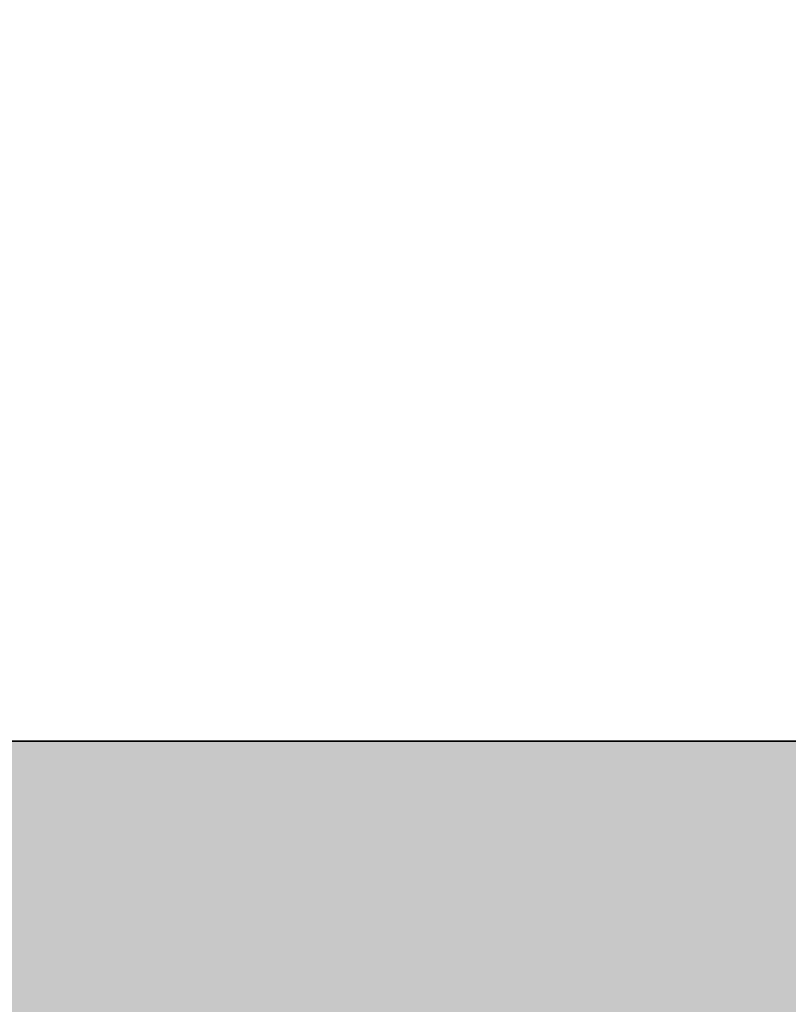
# Model space of a CAD drawing. Units: inches. Extents: x 2696 to 3240, y 1564 to 2310.
# Tile 72 of 76: x 3156.71 to 3168.22, y 2070.76 to 2085.5. Entities that reach past the tile are written whole.
import ezdxf

# ---------------------------------------------------------------- set-up
doc = ezdxf.new("R2010")
doc.units = ezdxf.units.IN
doc.layers.add('A-WALL', color=7, linetype='Continuous', lineweight=35)
doc.layers.add('A-WALL-PATT', color=9, linetype='Continuous', lineweight=13)

msp = doc.modelspace()

# ---------------------------------------------------------------- hatches: boundary and pattern name
at = {"layer": 'A-WALL-PATT', "transparency": 33554556}
h = msp.add_hatch(color=256, dxfattribs=at)
h.dxf.hatch_style = 1
h.paths.add_polyline_path([(2879.111, 2253.201), (2905.91, 2253.201), (2905.91, 2262.201), (2841.889, 2262.201), (2841.889, 2253.201), (2870.111, 2253.201), (2870.111, 2176.601), (2965.709, 2176.601), (2965.709, 2206.701), (2973.583, 2206.701), (2973.583, 2215.701), (2965.709, 2215.701), (2965.709, 2262.201), (2929.91, 2262.201), (2929.91, 2253.201), (2956.709, 2253.201), (2956.709, 2185.601), (2879.111, 2185.601)])
h.paths.add_polyline_path([(2782.834, 2262.201), (2745.611, 2262.201), (2745.611, 2228.729), (2754.611, 2228.729), (2754.611, 2253.201), (2782.834, 2253.201)])
h.paths.add_polyline_path([(2754.611, 2136.201), (2965.709, 2136.201), (2965.709, 2145.201), (2879.111, 2145.201), (2879.111, 2147.074), (2877.34, 2147.074), (2870.111, 2147.074), (2870.111, 2145.201), (2754.611, 2145.201), (2754.611, 2169.674), (2745.611, 2169.674), (2745.611, 2000.201), (2754.611, 2000.201), (2754.611, 2019.201), (2849.083, 2019.201), (2849.083, 2023.701), (2841.209, 2023.701), (2841.209, 2051.827), (2836.709, 2051.827), (2836.709, 2023.701), (2754.611, 2023.701), (2754.611, 2091.201), (2836.709, 2091.201), (2836.709, 2087.827), (2841.209, 2087.827), (2841.209, 2095.701), (2754.611, 2095.701)])
h.paths.add_polyline_path([(2965.709, 2136.201), (2956.709, 2136.201), (2956.709, 2023.701), (2885.083, 2023.701), (2885.083, 2019.201), (2956.709, 2019.201), (2956.709, 1950.575), (2965.709, 1950.575), (2965.709, 1980.201), (2973.583, 1980.201), (2973.583, 1989.201), (2965.709, 1989.201)])
h.paths.add_polyline_path([(2754.611, 1906.701), (2880.209, 1906.701), (2884.709, 1906.701), (2956.709, 1906.701), (2956.709, 1792.701), (2944.709, 1792.701), (2944.709, 1783.701), (2956.709, 1783.701), (2956.709, 1740.201), (2884.709, 1740.201), (2884.709, 1783.701), (2896.709, 1783.701), (2896.709, 1792.701), (2884.709, 1792.701), (2884.709, 1846.701), (2880.209, 1846.701), (2880.209, 1740.201), (2754.611, 1740.201), (2754.611, 1777.201), (2745.611, 1777.201), (2745.611, 1692.701), (2754.611, 1692.701), (2754.611, 1731.201), (2956.709, 1731.201), (2956.709, 1723.327), (2965.709, 1723.327), (2965.709, 1884.201), (2973.583, 1884.201), (2973.583, 1893.201), (2965.709, 1893.201), (2965.709, 1914.575), (2956.709, 1914.575), (2956.709, 1911.201), (2754.611, 1911.201), (2754.611, 1930.201), (2745.611, 1930.201), (2745.611, 1817.201), (2754.611, 1817.201), (2754.611, 1854.201), (2826.611, 1854.201), (2826.611, 1868.827), (2822.111, 1868.827), (2822.111, 1858.701), (2754.611, 1858.701)])
h.paths.add_polyline_path([(2965.709, 1656.201), (3008.237, 1656.201), (3008.237, 1665.201), (2965.709, 1665.201), (2965.709, 1693.327), (2956.709, 1693.327), (2956.709, 1686.201), (2934.583, 1686.201), (2934.583, 1681.701), (2956.709, 1681.701), (2956.709, 1614.201), (2896.709, 1614.201), (2896.709, 1681.701), (2904.583, 1681.701), (2904.583, 1686.201), (2892.209, 1686.201), (2892.209, 1614.201), (2858.41, 1614.201), (2858.41, 1605.201), (2965.709, 1605.201)])
h.paths.add_polyline_path([(2788.41, 1614.201), (2754.611, 1614.201), (2754.611, 1652.701), (2745.611, 1652.701), (2745.611, 1605.201), (2788.41, 1605.201)])
h.paths.add_polyline_path([(3199.611, 1633.048), (3190.611, 1633.048), (3190.611, 1614.201), (3082.611, 1614.201), (3082.611, 1665.201), (3070.237, 1665.201), (3070.237, 1656.201), (3078.111, 1656.201), (3078.111, 1605.201), (3199.611, 1605.201)])
h.paths.add_polyline_path([(3199.611, 1702.048), (3190.611, 1702.048), (3190.611, 1699.701), (3106.611, 1699.701), (3106.611, 1747.701), (3190.611, 1747.701), (3190.611, 1752.201), (3082.611, 1752.201), (3082.611, 1760.075), (3078.111, 1760.075), (3078.111, 1747.701), (3102.111, 1747.701), (3102.111, 1699.701), (3078.111, 1699.701), (3078.111, 1695.201), (3190.611, 1695.201), (3190.611, 1676.355), (3199.611, 1676.355)])
h.paths.add_polyline_path([(3199.611, 1783.201), (3190.611, 1783.201), (3190.611, 1745.355), (3199.611, 1745.355)])
h.paths.add_polyline_path([(3082.611, 1884.201), (3190.611, 1884.201), (3190.611, 1853.201), (3199.611, 1853.201), (3199.611, 1901.701), (3190.611, 1901.701), (3190.611, 1893.201), (3005.583, 1893.201), (3005.583, 1891.281), (3005.583, 1884.201), (3078.111, 1884.201), (3078.111, 1792.075), (3082.611, 1792.075)])
h.paths.add_polyline_path([(3199.611, 1994.701), (3190.611, 1994.701), (3190.611, 1989.201), (3073.709, 1989.201), (3073.709, 2034.201), (3069.209, 2034.201), (3069.209, 1989.201), (3005.583, 1989.201), (3005.583, 1980.201), (3190.611, 1980.201), (3190.611, 1971.701), (3199.611, 1971.701)])
h.paths.add_polyline_path([(3199.611, 2155.201), (3190.611, 2155.201), (3190.611, 2064.701), (3199.611, 2064.701)])
h.paths.add_polyline_path([(3190.611, 2074.701), (3106.611, 2074.701), (3106.611, 2122.701), (3190.611, 2122.701), (3190.611, 2127.201), (3082.709, 2127.201), (3082.709, 2135.075), (3073.709, 2135.075), (3073.709, 2122.701), (3102.111, 2122.701), (3102.111, 2074.701), (3069.209, 2074.701), (3069.209, 2070.201), (3190.611, 2070.201)])
h.paths.add_polyline_path([(3082.709, 2253.201), (3190.611, 2253.201), (3190.611, 2225.201), (3199.611, 2225.201), (3199.611, 2262.201), (3073.709, 2262.201), (3073.709, 2215.701), (3035.583, 2215.701), (3035.583, 2206.701), (3073.709, 2206.701), (3073.709, 2171.075), (3082.709, 2171.075)])

# ---------------------------------------------------------------- linework, layer by layer
at = {"layer": 'A-WALL'}
msp.add_line((3106.611, 2074.701), (3190.611, 2074.701), dxfattribs=at)

doc.saveas('drawing.dxf')
